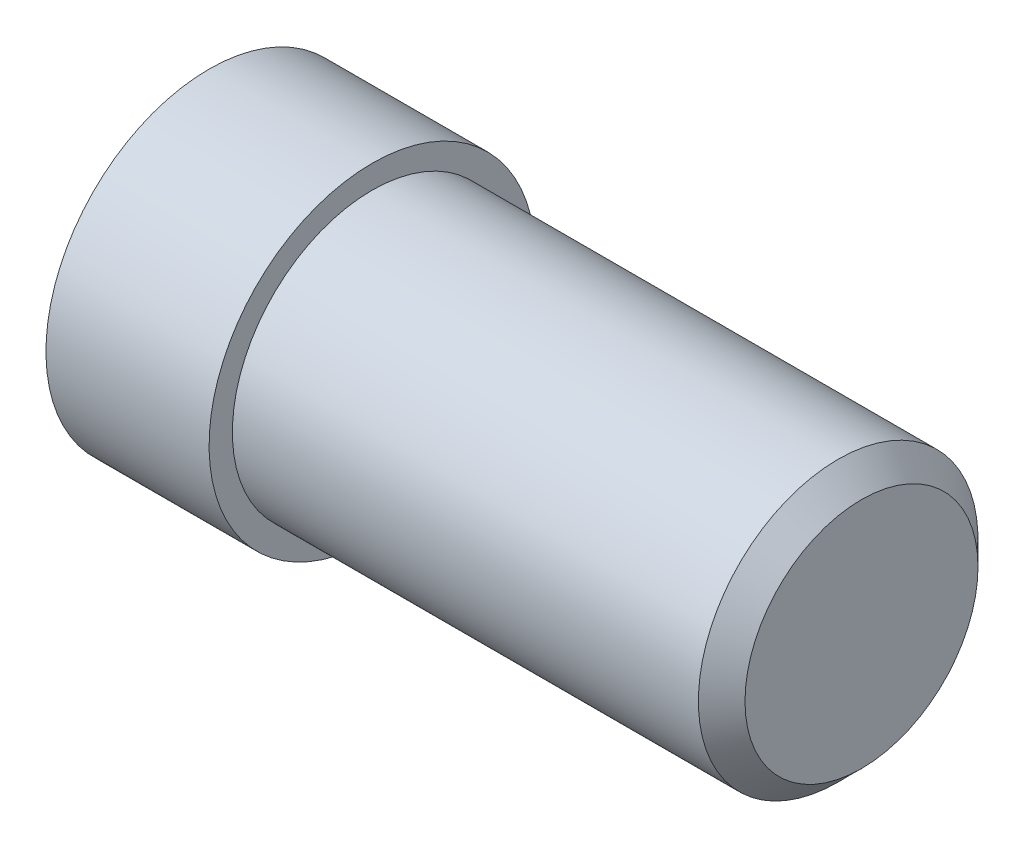
SolidWorks part; units mm, degrees
material "Plain Carbon Steel"
ref_plane "Front Plane" through (0, 0, 0) normal (0, 0, 1) x (1, 0, 0)
ref_plane "Top Plane" through (0, 0, 0) normal (0, 1, 0) x (1, 0, 0)
ref_plane "Right Plane" through (0, 0, 0) normal (1, 0, 0) x (0, 0, -1)
sketch "Bolt Profile Sketch" plane through (0, 0, 0) normal (0, 0, 1) x (1, 0, 0)
  line L0 (0, 0) -> (0, 6)
  line L1 (0, 6) -> (-21, 6)
  line L2 (-21, 6) -> (-21, 7)
  line L3 (-21, 7) -> (-28, 7)
  line L4 (-28, 7) -> (-28, 0)
  line L5 (0, 0) -> (-28, 0)
  dimension "D1" = 6
  dimension "D2" = 7
  dimension "D3" = 21
  dimension "D4" = 7
revolve "Bolt Body Revolve" add sketch "Bolt Profile Sketch" angle 360 about L5
chamfer "Shank End Chamfer 1x45" distance 1 angle 45 1 edges at (0, 6, 0)
